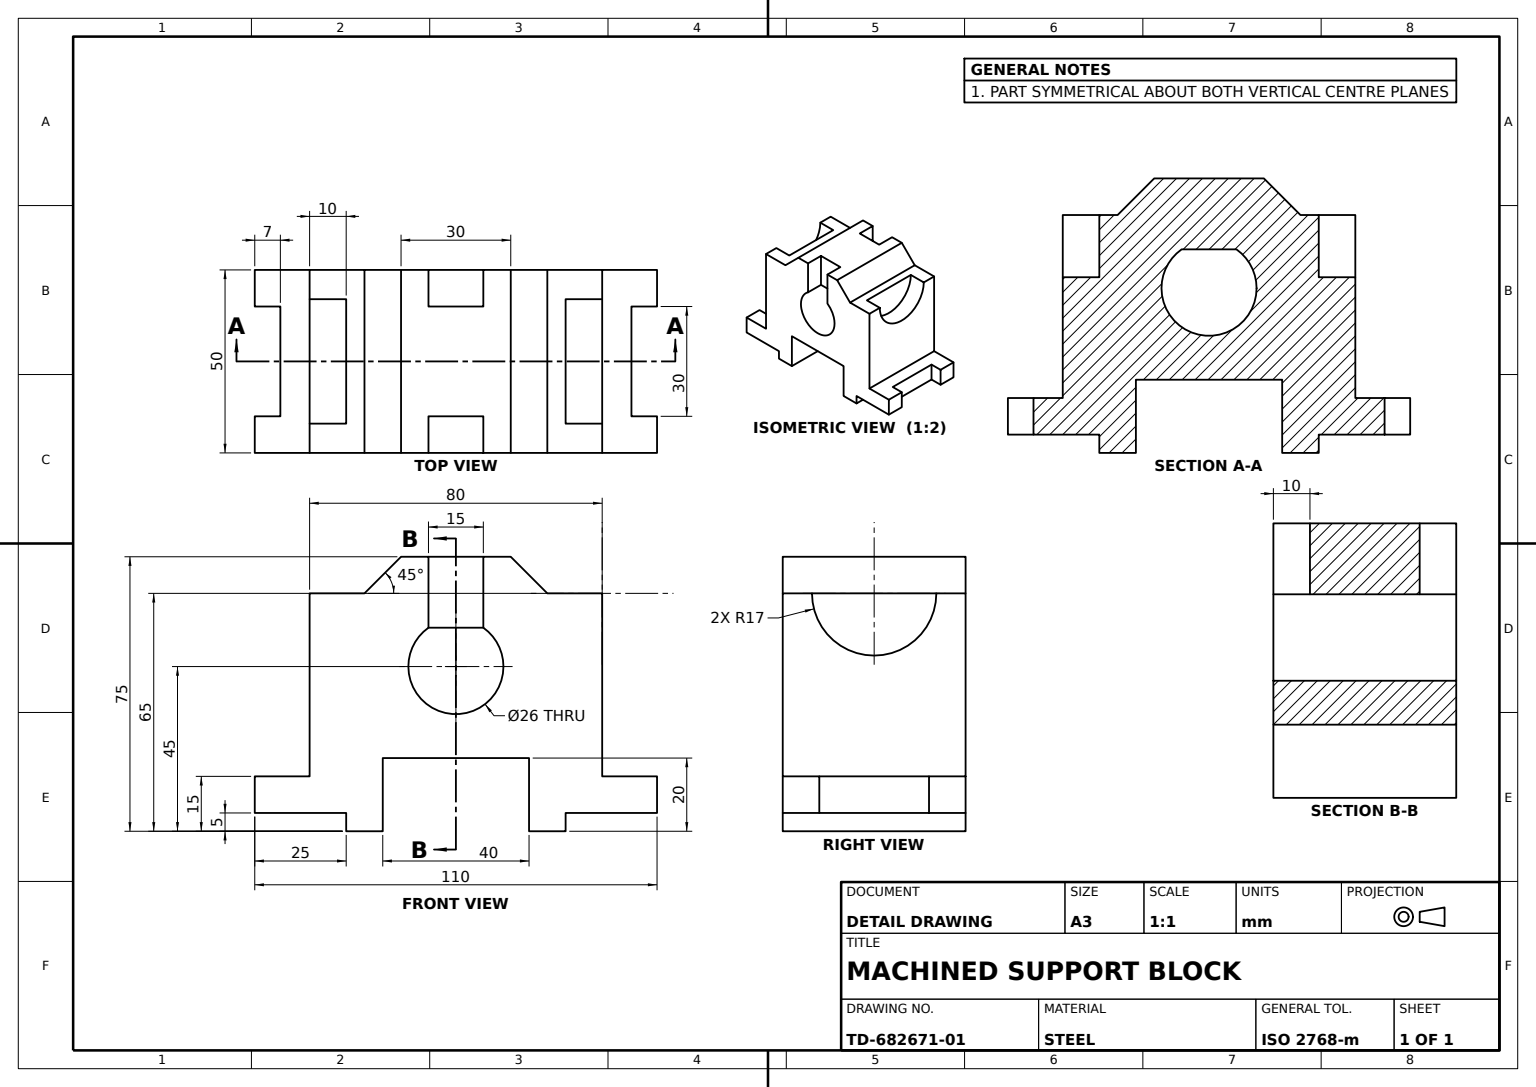
SolidWorks part; units mm, degrees
material "Plain Carbon Steel"
ref_plane "Front Plane" through (0, 0, 0) normal (0, 0, 1) x (1, 0, 0)
ref_plane "Top Plane" through (0, 0, 0) normal (0, 1, 0) x (1, 0, 0)
ref_plane "Right Plane" through (0, 0, 0) normal (1, 0, 0) x (0, 0, -1)
sketch "Stepped Block Profile" plane through (0, 0, 0) normal (1, 0, 0) x (0, 0, -1)
  line L0 (-20, -25) -> (20, -25)
  line L1 (20, -25) -> (20, -45)
  line L2 (20, -45) -> (30, -45)
  line L3 (30, -45) -> (30, -40)
  line L4 (30, -40) -> (55, -40)
  line L5 (55, -40) -> (55, -30)
  line L6 (55, -30) -> (40, -30)
  line L7 (40, -30) -> (40, 20)
  line L8 (40, 20) -> (25, 20)
  line L9 (25, 20) -> (15, 30)
  line L10 (15, 30) -> (7.5, 30)
  line L11 (7.5, 30) -> (7.5, 10.6184)
  line L12 (0, 0) -> (0, 13) construction
  line L13 (-7.5, 30) -> (-7.5, 10.6184)
  line L14 (-15, 30) -> (-7.5, 30)
  line L15 (-25, 20) -> (-15, 30)
  line L16 (-40, 20) -> (-25, 20)
  line L17 (-40, -30) -> (-40, 20)
  line L18 (-55, -30) -> (-40, -30)
  line L19 (-55, -40) -> (-55, -30)
  line L20 (-30, -40) -> (-55, -40)
  line L21 (-30, -45) -> (-30, -40)
  line L22 (-20, -45) -> (-30, -45)
  line L23 (-20, -25) -> (-20, -45)
  arc A0 (-7.5, 10.6184) -> (7.5, 10.6184) centre (0, 0) ccw
  point P28 (0, -25)
  point P30 (-25, -45)
  dimension "D1" = 26
  dimension "D2" = 45
  dimension "D3" = 5
  dimension "D4" = 20
  dimension "D5" = 25
  dimension "D6" = 40
  dimension "D7" = 110
  dimension "D8" = 10
  dimension "D9" = 15
  dimension "D10" = 65
  dimension "D11" = 75
  dimension "D12" = 80
  dimension "D13" = 50
  dimension "D14" = 30
extrude "Stepped Block Body 50mm" add sketch "Stepped Block Profile" along normal mid plane 50
sketch "End Slot Profile 30mm" plane through (0, 0, 55) normal (0, 0, 1) x (1, 0, 0)
  line L0 (25, -30) -> (-25, -30) construction
  line L1 (-15, -30) -> (15, -30)
  line L2 (-15, -30) -> (-15, -40)
  line L3 (-15, -40) -> (15, -40)
  line L4 (15, -30) -> (15, -40)
  line L5 (25, -40) -> (-25, -40) construction
  point P8 (0, -40)
  dimension "D1" = 30
extrude "End Slot Cut 7 Deep" cut sketch "End Slot Profile 30mm" against normal blind 7
sketch "Half Bore Profile" plane through (0, 0, 40) normal (0, 0, 1) x (1, 0, 0)
  line L0 (25, 20) -> (-25, 20) construction
  line L1 (-17, 20) -> (17, 20)
  arc A0 (-17, 20) -> (17, 20) centre (0, 20) ccw
  dimension "D1" = 17
extrude "Half Bore Cut 10 Deep" cut sketch "Half Bore Profile" against normal blind 10
mirror "End Slot and Bore Mirror" about plane through (0, 0, 0) normal (0, 0, 1) of "End Slot Cut 7 Deep", "Half Bore Cut 10 Deep"
sketch "Centre Boss Profile" plane through (0, 0, 0) normal (1, 0, 0) x (0, 0, -1)
  line L1 (-7.5, 30) -> (7.5, 30)
  line L2 (-7.5, 30) -> (-7.5, 10.6184)
  line L3 (-7.5, 10.6184) -> (7.5, 10.6184)
  line L4 (7.5, 30) -> (7.5, 10.6184)
extrude "Centre Boss 30mm" add sketch "Centre Boss Profile" along normal mid plane 30
